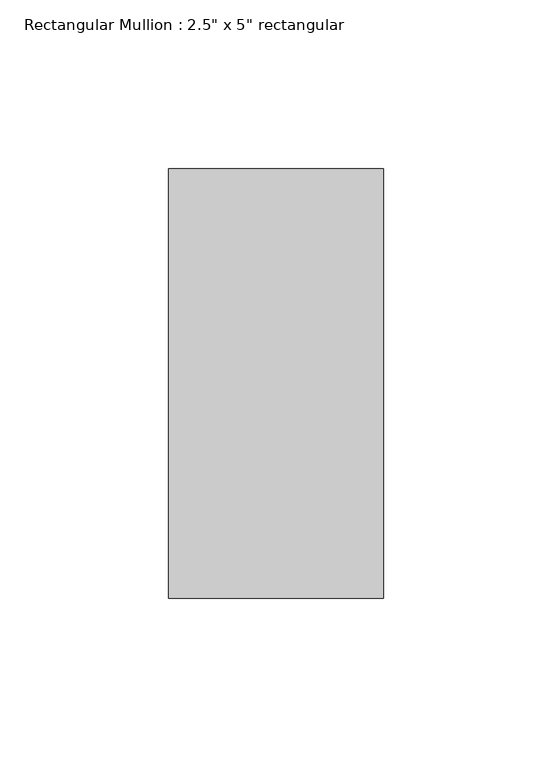
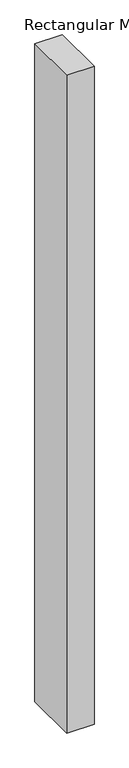
"""IFC4 building model written with IfcOpenShell, lengths in millimetres: member geometry."""

from ifc_helpers import new_model, si_unit, frame, origin, place, context, project, spatial, polyline, outline, extrude, source, transform, mapped, element, save


def member_6d802792(model_context):
    return source(origin(), model_context, "Body", "SweptSolid", [
        extrude(outline(polyline([(0.0, 63.5), (0.0, -63.5), (-63.5, -63.5), (-63.5, 63.5), (0.0, 63.5)])), frame((0.0, 0.0, -1608.6208916), z_axis=(0.0, 0.0, 1.0), x_axis=(1.0, 0.0, 0.0)), (0.0, 0.0, 1.0), 1608.6208916),
    ])


if __name__ == "__main__":
    model = new_model("IFC4")
    model_context = context("Model", 3, world=origin())
    ifc_project = project(units=[si_unit("LENGTHUNIT", "METRE", prefix="MILLI")], contexts=[model_context])
    site = spatial("IfcSite", under=ifc_project)
    building = spatial("IfcBuilding", under=site)
    placement = place(None, origin())
    member_shape = member_6d802792(model_context)
    element("IfcMember", 1, ObjectType="Rectangular Mullion : 2.5\" x 5\" rectangular", at=placement, inside=building, context=model_context, shape_type="MappedRepresentation", body=[
        mapped(member_shape, transform((0.0, 0.0, 0.0), x_axis=(1.0, 0.0, 0.0), y_axis=(0.0, 1.0, 0.0), z_axis=(0.0, 0.0, 1.0))),
    ])
    save(model, "model.ifc")

# Revit data of these elements
# Type "Rectangular Mullion : 2.5\" x 5\" rectangular"
#   built-in parameter 1007304 = 0.416667 (stored number, unit not read)
#   built-in parameter 1007301 = 0.104167 (stored number, unit not read)
#   built-in parameter 1007300 = 0.104167 (stored number, unit not read)
# Element 1 (IfcMember, "Rectangular Mullion : 2.5\" x 5\" rectangular")
#   Materials on its faces: "Aluminum"
# Materials
#   "Aluminum": class "Metal", colour RGB 247 247 247, transparency 0, Description = "Aluminum 6061", Cost = 0
